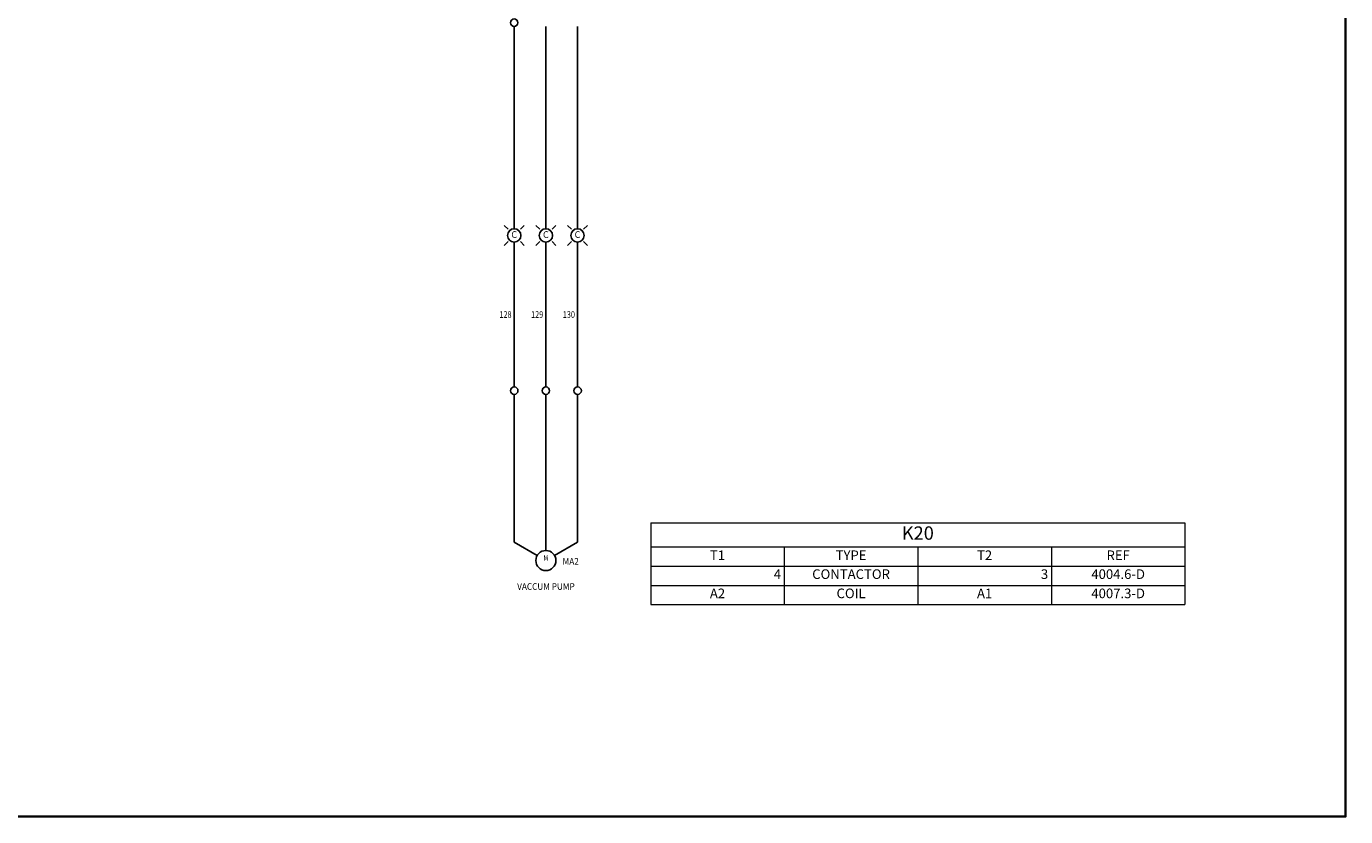
# Model space of a CAD drawing. Units: inches. Extents: x 12.5 to 62, y 4.7 to 37.4.
# Tile 4 of 5: x 37.3 to 62, y 4.7 to 19.5. Entities that reach past the tile are written whole.
import ezdxf
from ezdxf.enums import TextEntityAlignment as Align

# ---------------------------------------------------------------- set-up
doc = ezdxf.new("R2010")
doc.units = ezdxf.units.IN
doc.header["$MEASUREMENT"] = 0
for name, color, linetype, lineweight in [('16AWG-BLU', 182, 'Continuous', 25), ('16AWG-GRNYEL', 60, 'Continuous', 25), ('16AWG-RED', 1, 'Continuous', 25), ('E-ANNO-TTLB', 7, 'Continuous', 35), ('SYMS', 7, 'Continuous', 25), ('WIRENO', 72, 'Continuous', 18), ('XREF', 7, 'Continuous', 18)]:
    doc.layers.add(name, color=color, linetype=linetype, lineweight=lineweight)
for name, color, linetype in [('DESC', 150, 'Continuous'), ('MISC', 7, 'Continuous'), ('TAGS', 150, 'Continuous')]:
    doc.layers.add(name, color=color, linetype=linetype)
doc.styles.get("Standard").update_dxf_attribs({"font": 'arial.ttf'})
doc.styles.add('WD', font='romans.shx')

# ---------------------------------------------------------------- blocks, each defined once
blk = doc.blocks.new('VT0_02')
blk.add_circle((0, 0), 0.0699)
at = {"style": 'WD', "flags": 1}
for tag, p in [('X4TERM01', (-0.07, 0)), ('X2TERM01', (0, 0.07)), ('X1TERM01', (0.07, 0)), ('X8TERM01', (0, -0.07))]:
    blk.add_attdef(tag, p, '', height=0.01, dxfattribs=at)
blk = doc.blocks.new('VMO13')
blk.add_circle((0, 0), 0.188)
at = {"style": 'WD'}
for tag, p, width in [('INST', (0.318, 0.263), 0.7), ('TAG1', (0.312, -0.079), 0.9), ('LOC', (0.318, 0.094), 0.7)]:
    blk.add_attdef(tag, p, '', height=0.125, dxfattribs=dict(at, width=width))
for tag, height, width, p in [('RATING1', 0.1, 0.8, (0, 0)), ('DESC1', 0.125, 0.9, (0.001, -0.549)), ('DESC2', 0.125, 0.9, (0.001, -0.706)), ('DESC3', 0.125, 0.9, (0.001, -0.862)), ('RATING3', 0.125, 0.8, (0.001, -1.018)), ('WDTAGALT', 0.125, 0.7, (0, -1.344)), ('RATING4', 0.125, 0.8, (0.001, -1.174))]:
    blk.add_attdef(tag, text='', height=height, dxfattribs=dict(at, width=width)).set_placement(p, align=Align.CENTER)
at = {"style": 'WD', "flags": 1}
for tag, p in [('X0TERM03', (-0.162, 0.094)), ('X2TERM02', (0, 0.188)), ('X0TERM01', (0.162, 0.094)), ('X0TERM04', (0.133, -0.133))]:
    blk.add_attdef(tag, p, '', height=0.0125, dxfattribs=at)
at = {"style": 'WD', "flags": 9}
for tag, p in [('ASSYCODE', (0, 0.125)), ('FAMILY', (-0.005, 0.17))]:
    blk.add_attdef(tag, text='', height=0.01, dxfattribs=at).set_placement(p, align=Align.CENTER)
at = {"style": 'WD', "flags": 1}
for tag, p in [('MFG', (0, 0.14)), ('CAT', (0, 0.159))]:
    blk.add_attdef(tag, text='', height=0.01, dxfattribs=at).set_placement(p, align=Align.MIDDLE)
at = {"style": 'WD', "width": 0.8}
blk.add_attdef('RATING2', text='', height=0.1, dxfattribs=at).set_placement((0, -0.031), align=Align.TOP_CENTER)
blk = doc.blocks.new('VLT1C')
for p, q in [((-0.115, 0.115), (-0.186, 0.186)), ((0.115, 0.115), (0.186, 0.186)), ((-0.115, -0.115), (-0.186, -0.186)), ((0.115, -0.115), (0.186, -0.186))]:
    blk.add_line(p, q)
blk.add_circle((0, 0), 0.125)
at = {"style": 'WD'}
for tag, height, flags, p in [('TERM01', 0.125, 8, (-0.031, 0.219)), ('FAMILY', 0.01, 9, (-0.219, -0.117)), ('MFG', 0.01, 9, (-0.221, -0.149)), ('CAT', 0.01, 9, (-0.221, -0.134))]:
    blk.add_attdef(tag, text='', height=height, dxfattribs=dict(at, flags=flags)).set_placement(p, align=Align.RIGHT)
blk.add_attdef('COLOR', text='', height=0.125, dxfattribs=at).set_placement((0, 0), align=Align.MIDDLE)
at = {"style": 'WD', "flags": 1}
for tag, p in [('X2TERM01', (0, 0.125)), ('X8TERM02', (0, -0.125))]:
    blk.add_attdef(tag, p, '', height=0.0125, dxfattribs=at)
at = {"style": 'WD'}
for tag, p, width in [('TAG1', (0.2, -0.098), 0.9), ('DESC1', (-0.256, -0.931), 0.9), ('WDTAGALT', (-0.25, -1.25), 0.7)]:
    blk.add_attdef(tag, p, '', height=0.125, dxfattribs=dict(at, width=width))
at = {"style": 'WD', "flags": 8}
blk.add_attdef('TERM02', text='', height=0.125, dxfattribs=at).set_placement((-0.031, -0.219), align=Align.TOP_RIGHT)
at = {"style": 'WD', "flags": 9}
blk.add_attdef('ASSYCODE', text='', height=0.01, dxfattribs=at).set_placement((-0.238, -0.097), align=Align.CENTER)
at = {"style": 'WD'}
for tag, width, p in [('INST', 0.7, (0.281, -0.147)), ('LOC', 0.7, (0.281, -0.317)), ('DESC2', 0.9, (-0.256, -0.963))]:
    blk.add_attdef(tag, text='', height=0.125, dxfattribs=dict(at, width=width)).set_placement(p, align=Align.TOP_LEFT)
blk = doc.blocks.new('WD_WNV')
at = {"style": 'WD', "width": 0.8}
blk.add_attdef('WIRENO', text='', height=0.125, dxfattribs=at).set_placement((-0.05, 0), align=Align.MIDDLE_RIGHT)
at = {"style": 'WD', "flags": 1}
for tag, p in [('W01USER', (-0.062, 0.094)), ('W02USER', (-0.062, 0.086)), ('W03USER', (-0.062, 0.078)), ('W04USER', (-0.062, 0.07)), ('W05USER', (-0.062, 0.062)), ('W06USER', (-0.062, 0.055)), ('W07USER', (-0.062, 0.047)), ('W08USER', (-0.062, 0.039)), ('W09USER', (-0.062, 0.031)), ('W10USER', (-0.062, 0.023))]:
    blk.add_attdef(tag, text='', height=0.005, dxfattribs=at).set_placement(p, align=Align.CENTER)
blk = doc.blocks.new('*T30')
at = {"layer": 'XREF', "transparency": 16777216}
for p, q in [((0, 0), (10, 0)), ((0, 0), (0, -1.533)), ((10, 0), (10, -1.533)), ((0, -0.453), (10, -0.453)), ((2.5, -0.453), (2.5, -1.533)), ((5, -0.453), (5, -1.533)), ((7.5, -0.453), (7.5, -1.533)), ((0, -0.813), (10, -0.813)), ((0, -1.173), (10, -1.173)), ((0, -1.533), (10, -1.533))]:
    blk.add_line(p, q, dxfattribs=at)
at = {"layer": 'XREF', "color": 0, "transparency": 16777216}
for s, insert, char_height, width, attachment_point in [('K20', (5, -0.227), 0.25, 9.88, 5), ('T1', (1.25, -0.633), 0.18, 2.38, 5), ('TYPE', (3.75, -0.633), 0.18, 2.38, 5), ('T2', (6.25, -0.633), 0.18, 2.38, 5), ('REF', (8.75, -0.633), 0.18, 2.38, 5), ('4', (2.44, -0.873), 0.18, 2.38, 3), ('CONTACTOR', (3.75, -0.873), 0.18, 2.38, 2), ('3', (7.44, -0.873), 0.18, 2.38, 3), ('4004.6-D', (8.75, -0.873), 0.18, 2.38, 2), ('A2', (1.25, -1.233), 0.18, 2.38, 2), ('COIL', (3.75, -1.233), 0.18, 2.38, 2), ('A1', (6.25, -1.233), 0.18, 2.38, 2), ('4007.3-D', (8.75, -1.233), 0.18, 2.38, 2)]:
    blk.add_mtext(s, dxfattribs=dict(at, insert=insert, char_height=char_height, width=width, attachment_point=attachment_point))

msp = doc.modelspace()

# ---------------------------------------------------------------- linework, layer by layer
at = {"layer": '16AWG-BLU'}
for p, q in [((47.656, 19.527), (47.656, 15.741)), ((47.656, 15.491), (47.656, 12.781)), ((47.656, 12.641), (47.656, 9.876)), ((47.656, 9.876), (47.225, 9.627))]:
    msp.add_line(p, q, dxfattribs=at)
at = {"layer": '16AWG-GRNYEL'}
for p, q in [((47.062, 19.527), (47.062, 15.741)), ((47.062, 15.491), (47.062, 12.781)), ((47.062, 12.641), (47.062, 9.721))]:
    msp.add_line(p, q, dxfattribs=at)
at = {"layer": '16AWG-RED'}
for p, q in [((46.469, 19.527), (46.469, 15.741)), ((46.469, 15.491), (46.469, 12.781)), ((46.469, 12.641), (46.469, 9.876)), ((46.469, 9.876), (46.9, 9.627))]:
    msp.add_line(p, q, dxfattribs=at)
at = {"layer": 'E-ANNO-TTLB'}
msp.add_lwpolyline([(12.524, 37.377), (62.033, 37.377), (62.033, 4.741), (12.524, 4.741)], close=True, dxfattribs=at)

# ---------------------------------------------------------------- block references
msp.add_blockref('*T30', (49.025, 10.241))
at = {"layer": 'SYMS'}
for p in [(46.469, 19.597), (46.47, 12.711), (47.062, 12.711), (47.656, 12.711)]:
    msp.add_blockref('VT0_02', p, dxfattribs=at)
ref = msp.add_blockref('VLT1C', (46.469, 15.616), dxfattribs=at)
ref.add_attrib('COLOR', 'C', dxfattribs={"layer": 'MISC', "height": 0.125, "style": 'WD'}).set_placement((46.469, 15.616), align=Align.MIDDLE)
ref = msp.add_blockref('VLT1C', (47.062, 15.616), dxfattribs=at)
ref.add_attrib('COLOR', 'C', dxfattribs={"layer": 'MISC', "height": 0.125, "style": 'WD'}).set_placement((47.062, 15.616), align=Align.MIDDLE)
ref = msp.add_blockref('VLT1C', (47.654, 15.616), dxfattribs=at)
ref.add_attrib('COLOR', 'C', dxfattribs={"layer": 'MISC', "height": 0.125, "style": 'WD'}).set_placement((47.654, 15.616), align=Align.MIDDLE)
ref = msp.add_blockref('VMO13', (47.062, 9.533), dxfattribs=at)
ref.add_attrib('RATING1', 'M', dxfattribs={"layer": 'MISC', "height": 0.1, "style": 'WD', "width": 0.8}).set_placement((47.062, 9.533), align=Align.CENTER)
ref.add_attrib('DESC1', 'VACCUM PUMP', dxfattribs={"layer": 'DESC', "height": 0.125, "style": 'WD', "width": 0.9}).set_placement((47.063, 8.984), align=Align.CENTER)
ref.add_attrib('TAG1', 'MA2', (47.375, 9.454), dxfattribs={"layer": 'TAGS', "height": 0.125, "style": 'WD', "width": 0.9})
at = {"layer": 'WIRENO'}
ref = msp.add_blockref('WD_WNV', (46.469, 14.136), dxfattribs=at)
ref.add_attrib('WIRENO', '128', dxfattribs={"linetype": 'Continuous', "height": 0.125, "style": 'WD', "width": 0.8}).set_placement((46.419, 14.136), align=Align.MIDDLE_RIGHT)
ref = msp.add_blockref('WD_WNV', (47.062, 14.136), dxfattribs=at)
ref.add_attrib('WIRENO', '129', dxfattribs={"linetype": 'Continuous', "height": 0.125, "style": 'WD', "width": 0.8}).set_placement((47.012, 14.136), align=Align.MIDDLE_RIGHT)
ref = msp.add_blockref('WD_WNV', (47.656, 14.136), dxfattribs=at)
ref.add_attrib('WIRENO', '130', dxfattribs={"linetype": 'Continuous', "height": 0.125, "style": 'WD', "width": 0.8}).set_placement((47.606, 14.136), align=Align.MIDDLE_RIGHT)

doc.saveas('drawing.dxf')
